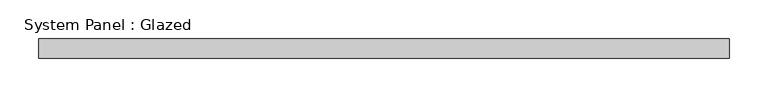
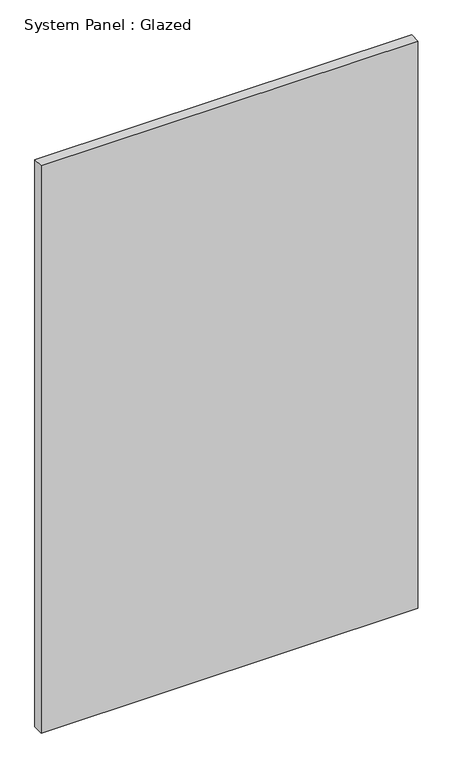
"""IFC4 building model written with IfcOpenShell, lengths in millimetres: plate geometry, System Panel : Glazed."""

from ifc_helpers import new_model, si_unit, origin, origin_with_axes, place, context, project, spatial, polyline, outline, extrude, source, transform, mapped, element, save


def system_panel_glazed_724d32f2(model_context):
    return source(origin(), model_context, "Body", "SweptSolid", [
        extrude(outline(polyline([(447.675, 19.05), (-447.675, 19.05), (-447.675, 44.45), (447.675, 44.45), (447.675, 19.05)])), origin_with_axes(), (0.0, 0.0, 1.0), 1424.6345763),
    ])


if __name__ == "__main__":
    model = new_model("IFC4")
    model_context = context("Model", 3, world=origin())
    ifc_project = project(units=[si_unit("LENGTHUNIT", "METRE", prefix="MILLI")], contexts=[model_context])
    site = spatial("IfcSite", under=ifc_project)
    building = spatial("IfcBuilding", under=site)
    placement = place(None, origin())
    system_panel_glazed_shape = system_panel_glazed_724d32f2(model_context)
    element("IfcPlate", 1, ObjectType="System Panel : Glazed", at=placement, inside=building, context=model_context, shape_type="MappedRepresentation", body=[
        mapped(system_panel_glazed_shape, transform((0.0, 0.0, 0.0), x_axis=(1.0, 0.0, 0.0), y_axis=(0.0, 1.0, 0.0), z_axis=(0.0, 0.0, 1.0))),
    ])
    save(model, "model.ifc")

# Revit data of these elements
# Type "System Panel : Glazed"
#   Construction Type Id = "GSP4R"
#   Analytic Construction = "1/8 in Pilkington single glazing"
#   Visual Light Transmittance = 0.9
#   Solar Heat Gain Coefficient = 0.86
#   Heat Transfer Coefficient (U) = 1.18115 BTU/(h·ft²·°F)
#   Define Thermal Properties by = 1
# Element 1 (IfcPlate, "System Panel : Glazed")
#   Materials on its faces: "Glass"
# Materials
#   "Glass": class "Glass", colour RGB 0 128 192, transparency 0.75, Description = "Soda Lime Glass", Cost = 0
